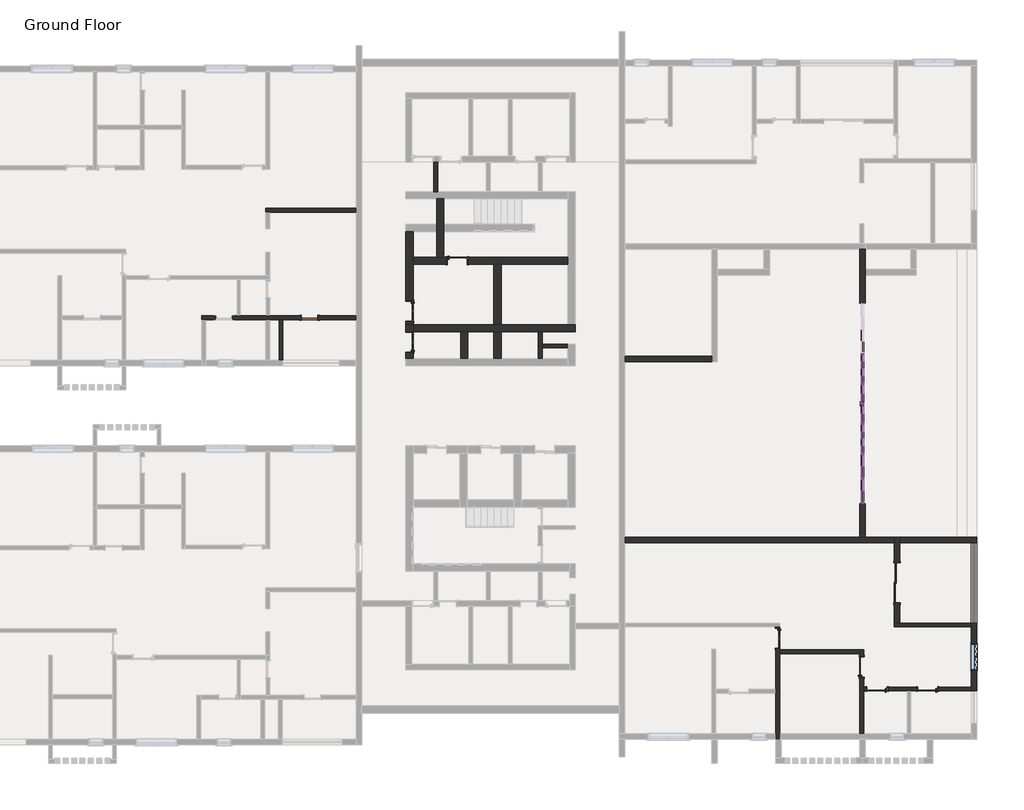
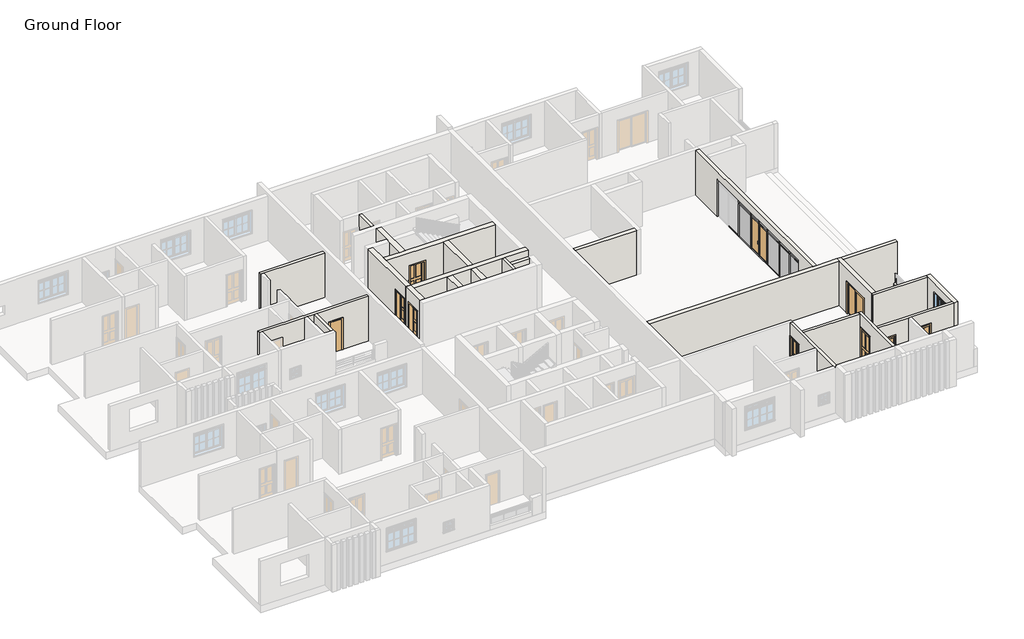
# One storey, part 4 of 9: 32 members, 26 walls, 10 doors, 10 plates, 1 window.
"""IFC4 building model written with IfcOpenShell, lengths in millimetres."""

from ifc_helpers import new_model, si_unit, origin, origin_with_axes, place, context, project, spatial, polyline, outline, extrude, faceted_brep, transform, mapped, element, save
from components import door_curtain_wall_double_storefront_door_curtain_wall_double_c727979e, door_double_sliding_6_7f701685, door_interior_single_4_panel_wood_3_x_7_bed_room_doors_9f8eaeea, door_interior_single_4_panel_wood_3_x_7_bed_room_doors_791c550c, door_interior_single_4_panel_wood_3_x_7_bed_room_doors_8c54f457, door_0af0cdd0, member_75d1e245, member_7db1855a, member_d2e7e466, member_80bb9b3a, member_1988fdfd, member_d37749d9, member_bf0a6844, member_74e81316, member_697f972d, member_78934672, member_3c3dc66a, member_222163d1, member_5cd4c5ac, member_860c46db, system_panel_glazed_fbb6c980, system_panel_glazed_ad1fd27a, system_panel_glazed_1d13bf28, system_panel_glazed_6ba3ac31, system_panel_glazed_eda788cd, system_panel_glazed_2483beae, system_panel_glazed_98578528, window_casement_double_awning_double_4_x_5_window_c6f36ef5

model = new_model("IFC4")

# Units and contexts
model_context = context("Model", 3, world=origin())
ifc_project = project(units=[si_unit("LENGTHUNIT", "METRE", prefix="MILLI")], contexts=[model_context])

# Site, building, storey
site = spatial("IfcSite", under=ifc_project)
building = spatial("IfcBuilding", under=site)
storey = spatial("IfcBuildingStorey", under=building, Name="Ground Floor", Elevation=0.0)

# Doors
placement = place(None, origin())
door_curtain_wall_double_storefront_door_curtain_wall_double_shape = door_curtain_wall_double_storefront_door_curtain_wall_double_c727979e(model_context)
element("IfcDoor", 1, ObjectType="Door-Curtain-Wall-Double-Storefront : Door-Curtain-Wall-Double-Storefront", at=placement, inside=storey, context=model_context, shape_type="MappedRepresentation", body=[
    mapped(door_curtain_wall_double_storefront_door_curtain_wall_double_shape, transform((26870.0546318, 13572.234892, 63.5), x_axis=(0.0, 1.0, 0.0), y_axis=(-1.0, 0.0, 0.0), z_axis=(0.0, 0.0, 1.0))),
])
door_double_sliding_6_shape = door_double_sliding_6_7f701685(model_context)
element("IfcDoor", 2, ObjectType="Door-Double-Sliding : 6'", at=placement, inside=storey, context=model_context, shape_type="MappedRepresentation", body=[
    mapped(door_double_sliding_6_shape, transform((28571.8546318, 5393.434892, 0.0), x_axis=(0.0, 1.0, 0.0), y_axis=(-1.0, 0.0, 0.0), z_axis=(0.0, 0.0, 1.0))),
])
door_interior_single_4_panel_wood_3_x_7_bed_room_doors_shape = door_interior_single_4_panel_wood_3_x_7_bed_room_doors_9f8eaeea(model_context)
element("IfcDoor", 3, ObjectType="Door-Interior-Single-4_Panel-Wood : 3' x 7' Bed Room Doors", at=placement, inside=storey, context=model_context, shape_type="MappedRepresentation", body=[
    mapped(door_interior_single_4_panel_wood_3_x_7_bed_room_doors_shape, transform((22999.7296318, 2866.134892, 0.0), x_axis=(0.0, -1.0, 0.0), y_axis=(1.0, 0.0, 0.0), z_axis=(0.0, 0.0, 1.0))),
])
element("IfcDoor", 4, ObjectType="Door-Interior-Single-4_Panel-Wood : 3' x 7' Bed Room Doors", at=placement, inside=storey, context=model_context, shape_type="MappedRepresentation", body=[
    mapped(door_interior_single_4_panel_wood_3_x_7_bed_room_doors_shape, transform((26828.7796318, 1558.034892, 0.0), x_axis=(0.0, 1.0, 0.0), y_axis=(-1.0, 0.0, 0.0), z_axis=(0.0, 0.0, 1.0))),
])
element("IfcDoor", 5, ObjectType="Door-Interior-Single-4_Panel-Wood : 3' x 7' Bed Room Doors", at=placement, inside=storey, context=model_context, shape_type="MappedRepresentation", body=[
    mapped(door_interior_single_4_panel_wood_3_x_7_bed_room_doors_shape, transform((27530.4546318, 551.559892, 0.0), x_axis=(-1.0, 0.0, 0.0), y_axis=(0.0, -1.0, 0.0), z_axis=(0.0, 0.0, 1.0))),
])
element("IfcDoor", 6, ObjectType="Door-Interior-Single-4_Panel-Wood : 3' x 7' Bed Room Doors", at=placement, inside=storey, context=model_context, shape_type="MappedRepresentation", body=[
    mapped(door_interior_single_4_panel_wood_3_x_7_bed_room_doors_shape, transform((29841.8546318, 551.559892, 0.0), x_axis=(-1.0, 0.0, 0.0), y_axis=(0.0, -1.0, 0.0), z_axis=(0.0, 0.0, 1.0))),
])
door_interior_single_4_panel_wood_3_x_7_bed_room_doors_2_shape = door_interior_single_4_panel_wood_3_x_7_bed_room_doors_791c550c(model_context)
element("IfcDoor", 7, ObjectType="Door-Interior-Single-4_Panel-Wood : 3' x 7' Bed Room Doors", at=placement, inside=storey, context=model_context, shape_type="MappedRepresentation", body=[
    mapped(door_interior_single_4_panel_wood_3_x_7_bed_room_doors_2_shape, transform((6210.3296318, 17788.634892, 0.0), x_axis=(0.0, -1.0, 0.0), y_axis=(1.0, 0.0, 0.0), z_axis=(0.0, 0.0, 1.0))),
])
element("IfcDoor", 8, ObjectType="Door-Interior-Single-4_Panel-Wood : 3' x 7' Bed Room Doors", at=placement, inside=storey, context=model_context, shape_type="MappedRepresentation", body=[
    mapped(door_interior_single_4_panel_wood_3_x_7_bed_room_doors_2_shape, transform((8378.8546318, 20090.509892, 0.0), x_axis=(1.0, 0.0, 0.0), y_axis=(0.0, 1.0, 0.0), z_axis=(0.0, 0.0, 1.0))),
])
door_interior_single_4_panel_wood_3_x_7_bed_room_doors_3_shape = door_interior_single_4_panel_wood_3_x_7_bed_room_doors_8c54f457(model_context)
element("IfcDoor", 9, ObjectType="Door-Interior-Single-4_Panel-Wood : 3' x 7' Bed Room Doors", at=placement, inside=storey, context=model_context, shape_type="MappedRepresentation", body=[
    mapped(door_interior_single_4_panel_wood_3_x_7_bed_room_doors_3_shape, transform((6210.3296318, 16366.234892, 0.0), x_axis=(0.0, 1.0, 0.0), y_axis=(-1.0, 0.0, 0.0), z_axis=(0.0, 0.0, 1.0))),
])
door_shape = door_0af0cdd0(model_context)
element("IfcDoor", 10, ObjectType="Single-Flush : 30\" x 80\"", at=placement, inside=storey, context=model_context, shape_type="MappedRepresentation", body=[
    mapped(door_shape, transform((1647.8546318, 17496.534892, 0.0), x_axis=(-1.0, 0.0, 0.0), y_axis=(0.0, -1.0, 0.0), z_axis=(0.0, 0.0, 1.0))),
])

# Members
member_shape = member_75d1e245(model_context)
element("IfcMember", 11, ObjectType="Rectangular Mullion : 2.5\" x 5\" rectangular", at=placement, inside=storey, context=model_context, shape_type="MappedRepresentation", body=[
    mapped(member_shape, transform((26870.0546318, 14486.634892, 2286.0), x_axis=(0.0, 1.0, 0.0), y_axis=(1.0, 0.0, 0.0), z_axis=(0.0, 0.0, -1.0))),
])
element("IfcMember", 12, ObjectType="Rectangular Mullion : 2.5\" x 5\" rectangular", at=placement, inside=storey, context=model_context, shape_type="MappedRepresentation", body=[
    mapped(member_shape, transform((26870.0546318, 12657.834892, 2286.0), x_axis=(0.0, 1.0, 0.0), y_axis=(1.0, 0.0, 0.0), z_axis=(0.0, 0.0, -1.0))),
])
element("IfcMember", 13, ObjectType="Rectangular Mullion : 2.5\" x 5\" rectangular", at=placement, inside=storey, context=model_context, shape_type="MappedRepresentation", body=[
    mapped(member_shape, transform((26870.0546318, 11286.234892, 2286.0), x_axis=(0.0, 1.0, 0.0), y_axis=(1.0, 0.0, 0.0), z_axis=(0.0, 0.0, -1.0))),
])
element("IfcMember", 14, ObjectType="Rectangular Mullion : 2.5\" x 5\" rectangular", at=placement, inside=storey, context=model_context, shape_type="MappedRepresentation", body=[
    mapped(member_shape, transform((26870.0546318, 10143.234892, 2286.0), x_axis=(0.0, 1.0, 0.0), y_axis=(1.0, 0.0, 0.0), z_axis=(0.0, 0.0, -1.0))),
])
element("IfcMember", 15, ObjectType="Rectangular Mullion : 2.5\" x 5\" rectangular", at=placement, inside=storey, context=model_context, shape_type="MappedRepresentation", body=[
    mapped(member_shape, transform((26870.0546318, 15858.234892, 2286.0), x_axis=(0.0, 1.0, 0.0), y_axis=(1.0, 0.0, 0.0), z_axis=(0.0, 0.0, -1.0))),
])
member_2_shape = member_7db1855a(model_context)
element("IfcMember", 16, ObjectType="Rectangular Mullion : 2.5\" x 5\" rectangular", at=placement, inside=storey, context=model_context, shape_type="MappedRepresentation", body=[
    mapped(member_2_shape, transform((26870.0546318, 13540.484892, 2286.0), x_axis=(0.0, 0.0, 1.0), y_axis=(1.0, 0.0, 0.0), z_axis=(0.0, 1.0, 0.0))),
])
element("IfcMember", 17, ObjectType="Rectangular Mullion : 2.5\" x 5\" rectangular", at=placement, inside=storey, context=model_context, shape_type="MappedRepresentation", body=[
    mapped(member_2_shape, transform((26870.0546318, 14454.884892, 2286.0), x_axis=(0.0, 0.0, 1.0), y_axis=(1.0, 0.0, 0.0), z_axis=(0.0, 1.0, 0.0))),
])
member_3_shape = member_d2e7e466(model_context)
element("IfcMember", 18, ObjectType="Rectangular Mullion : 2.5\" x 5\" rectangular", at=placement, inside=storey, context=model_context, shape_type="MappedRepresentation", body=[
    mapped(member_3_shape, transform((26870.0546318, 14454.884892, 2590.8), x_axis=(0.0, 0.0, 1.0), y_axis=(1.0, 0.0, 0.0), z_axis=(0.0, 1.0, 0.0))),
])
element("IfcMember", 19, ObjectType="Rectangular Mullion : 2.5\" x 5\" rectangular", at=placement, inside=storey, context=model_context, shape_type="MappedRepresentation", body=[
    mapped(member_3_shape, transform((26870.0546318, 13540.484892, 2590.8), x_axis=(0.0, 0.0, 1.0), y_axis=(1.0, 0.0, 0.0), z_axis=(0.0, 1.0, 0.0))),
])
member_4_shape = member_80bb9b3a(model_context)
element("IfcMember", 20, ObjectType="Rectangular Mullion : 2.5\" x 5\" rectangular", at=placement, inside=storey, context=model_context, shape_type="MappedRepresentation", body=[
    mapped(member_4_shape, transform((26870.0546318, 13572.234892, 2254.25), x_axis=(0.0, 1.0, 0.0), y_axis=(1.0, 0.0, 0.0), z_axis=(0.0, 0.0, -1.0))),
])
member_5_shape = member_1988fdfd(model_context)
element("IfcMember", 21, ObjectType="Rectangular Mullion : 2.5\" x 5\" rectangular", at=placement, inside=storey, context=model_context, shape_type="MappedRepresentation", body=[
    mapped(member_5_shape, transform((26870.0546318, 15826.484892, 2286.0), x_axis=(0.0, 0.0, 1.0), y_axis=(1.0, 0.0, 0.0), z_axis=(0.0, 1.0, 0.0))),
])
element("IfcMember", 22, ObjectType="Rectangular Mullion : 2.5\" x 5\" rectangular", at=placement, inside=storey, context=model_context, shape_type="MappedRepresentation", body=[
    mapped(member_5_shape, transform((26870.0546318, 12626.084892, 2286.0), x_axis=(0.0, 0.0, 1.0), y_axis=(1.0, 0.0, 0.0), z_axis=(0.0, 1.0, 0.0))),
])
member_6_shape = member_d37749d9(model_context)
element("IfcMember", 23, ObjectType="Rectangular Mullion : 2.5\" x 5\" rectangular", at=placement, inside=storey, context=model_context, shape_type="MappedRepresentation", body=[
    mapped(member_6_shape, transform((26870.0546318, 12626.084892, 2590.8), x_axis=(0.0, 0.0, 1.0), y_axis=(1.0, 0.0, 0.0), z_axis=(0.0, 1.0, 0.0))),
])
element("IfcMember", 24, ObjectType="Rectangular Mullion : 2.5\" x 5\" rectangular", at=placement, inside=storey, context=model_context, shape_type="MappedRepresentation", body=[
    mapped(member_6_shape, transform((26870.0546318, 15826.484892, 2590.8), x_axis=(0.0, 0.0, 1.0), y_axis=(1.0, 0.0, 0.0), z_axis=(0.0, 1.0, 0.0))),
])
member_7_shape = member_bf0a6844(model_context)
element("IfcMember", 25, ObjectType="Rectangular Mullion : 2.5\" x 5\" rectangular", at=placement, inside=storey, context=model_context, shape_type="MappedRepresentation", body=[
    mapped(member_7_shape, transform((26870.0546318, 11254.484892, 2286.0), x_axis=(0.0, 0.0, 1.0), y_axis=(1.0, 0.0, 0.0), z_axis=(0.0, 1.0, 0.0))),
])
member_8_shape = member_74e81316(model_context)
element("IfcMember", 26, ObjectType="Rectangular Mullion : 2.5\" x 5\" rectangular", at=placement, inside=storey, context=model_context, shape_type="MappedRepresentation", body=[
    mapped(member_8_shape, transform((26870.0546318, 11254.484892, 2590.8), x_axis=(0.0, 0.0, 1.0), y_axis=(1.0, 0.0, 0.0), z_axis=(0.0, 1.0, 0.0))),
])
member_9_shape = member_697f972d(model_context)
element("IfcMember", 27, ObjectType="Rectangular Mullion : 2.5\" x 5\" rectangular", at=placement, inside=storey, context=model_context, shape_type="MappedRepresentation", body=[
    mapped(member_9_shape, transform((26870.0546318, 10111.484892, 2286.0), x_axis=(0.0, 0.0, 1.0), y_axis=(1.0, 0.0, 0.0), z_axis=(0.0, 1.0, 0.0))),
])
member_10_shape = member_78934672(model_context)
element("IfcMember", 28, ObjectType="Rectangular Mullion : 2.5\" x 5\" rectangular", at=placement, inside=storey, context=model_context, shape_type="MappedRepresentation", body=[
    mapped(member_10_shape, transform((26870.0546318, 10111.484892, 2590.8), x_axis=(0.0, 0.0, 1.0), y_axis=(1.0, 0.0, 0.0), z_axis=(0.0, 1.0, 0.0))),
])
member_11_shape = member_3c3dc66a(model_context)
element("IfcMember", 29, ObjectType="Rectangular Mullion : 2.5\" x 5\" rectangular", at=placement, inside=storey, context=model_context, shape_type="MappedRepresentation", body=[
    mapped(member_11_shape, transform((26870.0546318, 9000.234892, 2590.8), x_axis=(0.0, -1.0, 0.0), y_axis=(1.0, 0.0, 0.0), z_axis=(0.0, 0.0, 1.0))),
])
member_12_shape = member_222163d1(model_context)
element("IfcMember", 30, ObjectType="Rectangular Mullion : 2.5\" x 5\" rectangular", at=placement, inside=storey, context=model_context, shape_type="MappedRepresentation", body=[
    mapped(member_12_shape, transform((26870.0546318, 14486.634892, 0.0), x_axis=(0.0, 1.0, 0.0), y_axis=(1.0, 0.0, 0.0), z_axis=(0.0, 0.0, -1.0))),
])
element("IfcMember", 31, ObjectType="Rectangular Mullion : 2.5\" x 5\" rectangular", at=placement, inside=storey, context=model_context, shape_type="MappedRepresentation", body=[
    mapped(member_12_shape, transform((26870.0546318, 12657.834892, 0.0), x_axis=(0.0, 1.0, 0.0), y_axis=(1.0, 0.0, 0.0), z_axis=(0.0, 0.0, -1.0))),
])
element("IfcMember", 32, ObjectType="Rectangular Mullion : 2.5\" x 5\" rectangular", at=placement, inside=storey, context=model_context, shape_type="MappedRepresentation", body=[
    mapped(member_12_shape, transform((26870.0546318, 11286.234892, 0.0), x_axis=(0.0, 1.0, 0.0), y_axis=(1.0, 0.0, 0.0), z_axis=(0.0, 0.0, -1.0))),
])
element("IfcMember", 33, ObjectType="Rectangular Mullion : 2.5\" x 5\" rectangular", at=placement, inside=storey, context=model_context, shape_type="MappedRepresentation", body=[
    mapped(member_12_shape, transform((26870.0546318, 10143.234892, 0.0), x_axis=(0.0, 1.0, 0.0), y_axis=(1.0, 0.0, 0.0), z_axis=(0.0, 0.0, -1.0))),
])
element("IfcMember", 34, ObjectType="Rectangular Mullion : 2.5\" x 5\" rectangular", at=placement, inside=storey, context=model_context, shape_type="MappedRepresentation", body=[
    mapped(member_12_shape, transform((26870.0546318, 15858.234892, 0.0), x_axis=(0.0, 1.0, 0.0), y_axis=(1.0, 0.0, 0.0), z_axis=(0.0, 0.0, -1.0))),
])
element("IfcMember", 35, ObjectType="Rectangular Mullion : 2.5\" x 5\" rectangular", at=placement, inside=storey, context=model_context, shape_type="MappedRepresentation", body=[
    mapped(member_8_shape, transform((26870.0546318, 10174.984892, 0.0), x_axis=(0.0, 0.0, -1.0), y_axis=(1.0, 0.0, 0.0), z_axis=(0.0, -1.0, 0.0))),
])
element("IfcMember", 36, ObjectType="Rectangular Mullion : 2.5\" x 5\" rectangular", at=placement, inside=storey, context=model_context, shape_type="MappedRepresentation", body=[
    mapped(member_8_shape, transform((26870.0546318, 15889.984892, 0.0), x_axis=(0.0, 0.0, -1.0), y_axis=(1.0, 0.0, 0.0), z_axis=(0.0, -1.0, 0.0))),
])
element("IfcMember", 37, ObjectType="Rectangular Mullion : 2.5\" x 5\" rectangular", at=placement, inside=storey, context=model_context, shape_type="MappedRepresentation", body=[
    mapped(member_6_shape, transform((26870.0546318, 14518.384892, 0.0), x_axis=(0.0, 0.0, -1.0), y_axis=(1.0, 0.0, 0.0), z_axis=(0.0, -1.0, 0.0))),
])
element("IfcMember", 38, ObjectType="Rectangular Mullion : 2.5\" x 5\" rectangular", at=placement, inside=storey, context=model_context, shape_type="MappedRepresentation", body=[
    mapped(member_6_shape, transform((26870.0546318, 11317.984892, 0.0), x_axis=(0.0, 0.0, -1.0), y_axis=(1.0, 0.0, 0.0), z_axis=(0.0, -1.0, 0.0))),
])
member_13_shape = member_5cd4c5ac(model_context)
element("IfcMember", 39, ObjectType="Rectangular Mullion : 2.5\" x 5\" rectangular", at=placement, inside=storey, context=model_context, shape_type="MappedRepresentation", body=[
    mapped(member_13_shape, transform((26870.0546318, 12689.584892, 0.0), x_axis=(0.0, 0.0, -1.0), y_axis=(1.0, 0.0, 0.0), z_axis=(0.0, -1.0, 0.0))),
])
element("IfcMember", 40, ObjectType="Rectangular Mullion : 2.5\" x 5\" rectangular", at=placement, inside=storey, context=model_context, shape_type="MappedRepresentation", body=[
    mapped(member_10_shape, transform((26870.0546318, 9063.734892, 0.0), x_axis=(0.0, 0.0, -1.0), y_axis=(1.0, 0.0, 0.0), z_axis=(0.0, -1.0, 0.0))),
])
element("IfcMember", 41, ObjectType="Rectangular Mullion : 2.5\" x 5\" rectangular", at=placement, inside=storey, context=model_context, shape_type="MappedRepresentation", body=[
    mapped(member_13_shape, transform((26870.0546318, 13572.234892, 0.0), x_axis=(0.0, 0.0, -1.0), y_axis=(1.0, 0.0, 0.0), z_axis=(0.0, -1.0, 0.0))),
])
member_14_shape = member_860c46db(model_context)
element("IfcMember", 42, ObjectType="Rectangular Mullion : 2.5\" x 5\" rectangular", at=placement, inside=storey, context=model_context, shape_type="MappedRepresentation", body=[
    mapped(member_14_shape, transform((26870.0546318, 9000.234892, 2286.0), x_axis=(0.0, -1.0, 0.0), y_axis=(1.0, 0.0, 0.0), z_axis=(0.0, 0.0, 1.0))),
])

# Plates
system_panel_glazed_shape = system_panel_glazed_fbb6c980(model_context)
element("IfcPlate", 43, ObjectType="System Panel : Glazed", at=placement, inside=storey, context=model_context, shape_type="MappedRepresentation", body=[
    mapped(system_panel_glazed_shape, transform((26870.0546318, 13115.034892, 2317.75), x_axis=(0.0, 1.0, 0.0), y_axis=(-1.0, 0.0, 0.0), z_axis=(0.0, 0.0, 1.0))),
])
element("IfcPlate", 44, ObjectType="System Panel : Glazed", at=placement, inside=storey, context=model_context, shape_type="MappedRepresentation", body=[
    mapped(system_panel_glazed_shape, transform((26870.0546318, 14029.434892, 2317.75), x_axis=(0.0, 1.0, 0.0), y_axis=(-1.0, 0.0, 0.0), z_axis=(0.0, 0.0, 1.0))),
])
system_panel_glazed_2_shape = system_panel_glazed_ad1fd27a(model_context)
element("IfcPlate", 45, ObjectType="System Panel : Glazed", at=placement, inside=storey, context=model_context, shape_type="MappedRepresentation", body=[
    mapped(system_panel_glazed_2_shape, transform((26870.0546318, 11972.034892, 2317.75), x_axis=(0.0, 1.0, 0.0), y_axis=(-1.0, 0.0, 0.0), z_axis=(0.0, 0.0, 1.0))),
])
element("IfcPlate", 46, ObjectType="System Panel : Glazed", at=placement, inside=storey, context=model_context, shape_type="MappedRepresentation", body=[
    mapped(system_panel_glazed_2_shape, transform((26870.0546318, 15172.434892, 2317.75), x_axis=(0.0, 1.0, 0.0), y_axis=(-1.0, 0.0, 0.0), z_axis=(0.0, 0.0, 1.0))),
])
system_panel_glazed_3_shape = system_panel_glazed_1d13bf28(model_context)
element("IfcPlate", 47, ObjectType="System Panel : Glazed", at=placement, inside=storey, context=model_context, shape_type="MappedRepresentation", body=[
    mapped(system_panel_glazed_3_shape, transform((26870.0546318, 10714.734892, 2317.75), x_axis=(0.0, 1.0, 0.0), y_axis=(-1.0, 0.0, 0.0), z_axis=(0.0, 0.0, 1.0))),
])
system_panel_glazed_4_shape = system_panel_glazed_6ba3ac31(model_context)
element("IfcPlate", 48, ObjectType="System Panel : Glazed", at=placement, inside=storey, context=model_context, shape_type="MappedRepresentation", body=[
    mapped(system_panel_glazed_4_shape, transform((26870.0546318, 9587.609892, 2317.75), x_axis=(0.0, 1.0, 0.0), y_axis=(-1.0, 0.0, 0.0), z_axis=(0.0, 0.0, 1.0))),
])
system_panel_glazed_5_shape = system_panel_glazed_eda788cd(model_context)
element("IfcPlate", 49, ObjectType="System Panel : Glazed", at=placement, inside=storey, context=model_context, shape_type="MappedRepresentation", body=[
    mapped(system_panel_glazed_5_shape, transform((26870.0546318, 9587.609892, 63.5), x_axis=(0.0, 1.0, 0.0), y_axis=(-1.0, 0.0, 0.0), z_axis=(0.0, 0.0, 1.0))),
])
system_panel_glazed_6_shape = system_panel_glazed_2483beae(model_context)
element("IfcPlate", 50, ObjectType="System Panel : Glazed", at=placement, inside=storey, context=model_context, shape_type="MappedRepresentation", body=[
    mapped(system_panel_glazed_6_shape, transform((26870.0546318, 11972.034892, 63.5), x_axis=(0.0, 1.0, 0.0), y_axis=(-1.0, 0.0, 0.0), z_axis=(0.0, 0.0, 1.0))),
])
element("IfcPlate", 51, ObjectType="System Panel : Glazed", at=placement, inside=storey, context=model_context, shape_type="MappedRepresentation", body=[
    mapped(system_panel_glazed_6_shape, transform((26870.0546318, 15172.434892, 63.5), x_axis=(0.0, 1.0, 0.0), y_axis=(-1.0, 0.0, 0.0), z_axis=(0.0, 0.0, 1.0))),
])
system_panel_glazed_7_shape = system_panel_glazed_98578528(model_context)
element("IfcPlate", 52, ObjectType="System Panel : Glazed", at=placement, inside=storey, context=model_context, shape_type="MappedRepresentation", body=[
    mapped(system_panel_glazed_7_shape, transform((26870.0546318, 10714.734892, 63.5), x_axis=(0.0, 1.0, 0.0), y_axis=(-1.0, 0.0, 0.0), z_axis=(0.0, 0.0, 1.0))),
])

# Walls
element("IfcWall", 53, ObjectType="12\" EXTERIOR WALL", at=placement, inside=storey, context=model_context, shape_type="Brep", body=[
    faceted_brep([(6372.2546318, 16848.834892, 0.0), (6372.2546318, 17179.034892, 0.0), (6372.2546318, 17179.034892, 3048.0), (6372.2546318, 16848.834892, 3048.0), (6372.2546318, 15629.634892, 3048.0), (6372.2546318, 15629.634892, 0.0), (6372.2546318, 15883.634892, 0.0), (6372.2546318, 15883.634892, 2159.0), (6372.2546318, 16848.834892, 2159.0), (6042.0546318, 17179.034892, 0.0), (6042.0546318, 16848.834892, 0.0), (6042.0546318, 16848.834892, 2159.0), (6042.0546318, 15883.634892, 2159.0), (6042.0546318, 15883.634892, 0.0), (6042.0546318, 15629.634892, 0.0), (6042.0546318, 15629.634892, 3048.0), (6042.0546318, 17179.034892, 3048.0)], [[[0, 1, 2, 3, 4, 5, 6, 7, 8]], [[9, 10, 11, 12, 13, 14, 15, 16]], [[5, 14, 13, 6]], [[9, 1, 0, 10]], [[14, 5, 4, 15]], [[1, 9, 16, 2]], [[4, 3, 2, 16, 15]], [[8, 11, 10, 0]], [[11, 8, 7, 12]], [[12, 7, 6, 13]]]),
])
element("IfcWall", 54, ObjectType="12\" EXTERIOR WALL", at=placement, inside=storey, context=model_context, shape_type="Brep", body=[
    faceted_brep([(6372.2546318, 16848.834892, 0.0), (8531.2546318, 16848.834892, 0.0), (8861.4546318, 16848.834892, 0.0), (10055.2546318, 16848.834892, 0.0), (10385.4546318, 16848.834892, 0.0), (12087.2546318, 16848.834892, 0.0), (12265.0546318, 16848.834892, 0.0), (13763.6546318, 16848.834892, 0.0), (13763.6546318, 16848.834892, 3048.0), (12265.0546318, 16848.834892, 3048.0), (12087.2546318, 16848.834892, 3048.0), (6372.2546318, 16848.834892, 3048.0), (13763.6546318, 17179.034892, 0.0), (13433.4546318, 17179.034892, 0.0), (10385.4546318, 17179.034892, 0.0), (10055.2546318, 17179.034892, 0.0), (6372.2546318, 17179.034892, 0.0), (6372.2546318, 17179.034892, 3048.0), (13763.6546318, 17179.034892, 3048.0)], [[[0, 1, 2, 3, 4, 5, 6, 7, 8, 9, 10, 11]], [[12, 13, 14, 15, 16, 17, 18]], [[7, 6, 5, 4, 3, 2, 1, 0, 16, 15, 14, 13, 12]], [[16, 0, 11, 17]], [[7, 12, 18, 8]], [[11, 10, 9, 8, 18, 17]]]),
])
element("IfcWall", 55, ObjectType="12\" EXTERIOR WALL", at=placement, inside=storey, context=model_context, shape_type="SweptSolid", body=[
    extrude(outline(polyline([(10055.2546318, 15629.634892), (10055.2546318, 16848.834892), (10385.4546318, 16848.834892), (10385.4546318, 15629.634892), (10055.2546318, 15629.634892)])), origin_with_axes(), (0.0, 0.0, 1.0), 3048.0),
])
element("IfcWall", 56, ObjectType="12\" EXTERIOR WALL", at=placement, inside=storey, context=model_context, shape_type="SweptSolid", body=[
    extrude(outline(polyline([(8531.2546318, 15629.634892), (8531.2546318, 16848.834892), (8861.4546318, 16848.834892), (8861.4546318, 15629.634892), (8531.2546318, 15629.634892)])), origin_with_axes(), (0.0, 0.0, 1.0), 3048.0),
])
element("IfcWall", 57, ObjectType="12\" EXTERIOR WALL", at=placement, inside=storey, context=model_context, shape_type="Brep", body=[
    faceted_brep([(13433.4546318, 20252.434892, 0.0), (8861.4546318, 20252.434892, 0.0), (8861.4546318, 20252.434892, 2159.0), (7896.2546318, 20252.434892, 2159.0), (7896.2546318, 20252.434892, 0.0), (7769.2546318, 20252.434892, 0.0), (7439.0546318, 20252.434892, 0.0), (6372.2546318, 20252.434892, 0.0), (6372.2546318, 20252.434892, 3048.0), (7439.0546318, 20252.434892, 3048.0), (7769.2546318, 20252.434892, 3048.0), (9166.2546318, 20252.434892, 3048.0), (13433.4546318, 20252.434892, 3048.0), (8861.4546318, 19922.234892, 0.0), (10055.2546318, 19922.234892, 0.0), (10385.4546318, 19922.234892, 0.0), (13433.4546318, 19922.234892, 0.0), (13433.4546318, 19922.234892, 3048.0), (10385.4546318, 19922.234892, 3048.0), (10055.2546318, 19922.234892, 3048.0), (6372.2546318, 19922.234892, 3048.0), (6372.2546318, 19922.234892, 0.0), (7896.2546318, 19922.234892, 0.0), (7896.2546318, 19922.234892, 2159.0), (8861.4546318, 19922.234892, 2159.0)], [[[0, 1, 2, 3, 4, 5, 6, 7, 8, 9, 10, 11, 12]], [[13, 14, 15, 16, 17, 18, 19, 20, 21, 22, 23, 24]], [[0, 16, 15, 14, 13, 1]], [[21, 7, 6, 5, 4, 22]], [[16, 0, 12, 17]], [[7, 21, 20, 8]], [[12, 11, 10, 9, 8, 20, 19, 18, 17]], [[24, 2, 1, 13]], [[2, 24, 23, 3]], [[3, 23, 22, 4]]]),
])
element("IfcWall", 58, ObjectType="12\" EXTERIOR WALL", at=placement, inside=storey, context=model_context, shape_type="SweptSolid", body=[
    extrude(outline(polyline([(10055.2546318, 17179.034892), (10055.2546318, 19922.234892), (10385.4546318, 19922.234892), (10385.4546318, 17179.034892), (10055.2546318, 17179.034892)])), origin_with_axes(), (0.0, 0.0, 1.0), 3048.0),
])
element("IfcWall", 59, ObjectType="12\" EXTERIOR WALL", at=placement, inside=storey, context=model_context, shape_type="Brep", body=[
    faceted_brep([(6042.0546318, 17306.034892, 0.0), (6042.0546318, 17179.034892, 0.0), (6042.0546318, 17179.034892, 3048.0), (6042.0546318, 21420.834892, 3048.0), (6042.0546318, 21420.834892, 0.0), (6042.0546318, 18271.234892, 0.0), (6042.0546318, 18271.234892, 2159.0), (6042.0546318, 17306.034892, 2159.0), (6372.2546318, 17179.034892, 0.0), (6372.2546318, 17306.034892, 0.0), (6372.2546318, 17306.034892, 2159.0), (6372.2546318, 18271.234892, 2159.0), (6372.2546318, 18271.234892, 0.0), (6372.2546318, 19922.234892, 0.0), (6372.2546318, 20252.434892, 0.0), (6372.2546318, 21420.834892, 0.0), (6372.2546318, 21420.834892, 3048.0), (6372.2546318, 20252.434892, 3048.0), (6372.2546318, 19922.234892, 3048.0), (6372.2546318, 17179.034892, 3048.0)], [[[0, 1, 2, 3, 4, 5, 6, 7]], [[8, 9, 10, 11, 12, 13, 14, 15, 16, 17, 18, 19]], [[8, 1, 0, 9]], [[4, 15, 14, 13, 12, 5]], [[1, 8, 19, 2]], [[15, 4, 3, 16]], [[3, 2, 19, 18, 17, 16]], [[7, 10, 9, 0]], [[10, 7, 6, 11]], [[11, 6, 5, 12]]]),
])
element("IfcWall", 60, ObjectType="12\" EXTERIOR WALL", at=placement, inside=storey, context=model_context, shape_type="Brep", body=[
    faceted_brep([(7439.0546318, 22919.434892, 0.0), (7439.0546318, 21751.034892, 0.0), (7439.0546318, 21420.834892, 0.0), (7439.0546318, 20252.434892, 0.0), (7439.0546318, 20252.434892, 3048.0), (7439.0546318, 21420.834892, 3048.0), (7439.0546318, 21751.034892, 3048.0), (7439.0546318, 22919.434892, 3048.0), (7769.2546318, 20252.434892, 0.0), (7769.2546318, 21420.834892, 0.0), (7769.2546318, 21751.034892, 0.0), (7769.2546318, 22919.434892, 0.0), (7769.2546318, 22919.434892, 3048.0), (7769.2546318, 21751.034892, 3048.0), (7769.2546318, 21420.834892, 3048.0), (7769.2546318, 20252.434892, 3048.0)], [[[0, 1, 2, 3, 4, 5, 6, 7]], [[8, 9, 10, 11, 12, 13, 14, 15]], [[3, 2, 1, 0, 11, 10, 9, 8]], [[3, 8, 15, 4]], [[7, 6, 5, 4, 15, 14, 13, 12]], [[11, 0, 7, 12]]]),
])
element("IfcWall", 61, ObjectType="6\" INTERIOR WALL", at=placement, inside=storey, context=model_context, shape_type="Brep", body=[
    faceted_brep([(12087.2546318, 16848.834892, 0.0), (12087.2546318, 15629.634892, 0.0), (12087.2546318, 15629.634892, 3048.0), (12087.2546318, 16848.834892, 3048.0), (12265.0546318, 15629.634892, 0.0), (12265.0546318, 16112.234892, 0.0), (12265.0546318, 16290.034892, 0.0), (12265.0546318, 16848.834892, 0.0), (12265.0546318, 16848.834892, 3048.0), (12265.0546318, 16290.034892, 3048.0), (12265.0546318, 16112.234892, 3048.0), (12265.0546318, 15629.634892, 3048.0)], [[[0, 1, 2, 3]], [[4, 5, 6, 7, 8, 9, 10, 11]], [[1, 0, 7, 6, 5, 4]], [[1, 4, 11, 2]], [[7, 0, 3, 8]], [[3, 2, 11, 10, 9, 8]]]),
])
element("IfcWall", 62, ObjectType="6\" INTERIOR WALL", at=placement, inside=storey, context=model_context, shape_type="SweptSolid", body=[
    extrude(outline(polyline([(12265.0546318, 16290.034892), (13433.4546318, 16290.034892), (13433.4546318, 16112.234892), (12265.0546318, 16112.234892), (12265.0546318, 16290.034892)])), origin_with_axes(), (0.0, 0.0, 1.0), 3048.0),
])
element("IfcWall", 63, ObjectType="6\" INTERIOR WALL", at=placement, inside=storey, context=model_context, shape_type="Brep", body=[
    faceted_brep([(-1882.7453682, 17585.434892, 0.0), (-1882.7453682, 17585.434892, 2133.6), (-2644.7453682, 17585.434892, 2133.6), (-2644.7453682, 17585.434892, 0.0), (-3279.7453682, 17585.434892, 0.0), (-3279.7453682, 17585.434892, 3048.0), (-1654.1453682, 17585.434892, 3048.0), (-1514.4453682, 17585.434892, 3048.0), (-320.6453682, 17585.434892, 3048.0), (-180.9453682, 17585.434892, 3048.0), (3781.4546318, 17585.434892, 3048.0), (3781.4546318, 17585.434892, 0.0), (2028.8546318, 17585.434892, 0.0), (2028.8546318, 17585.434892, 2133.6), (1266.8546318, 17585.434892, 2133.6), (1266.8546318, 17585.434892, 0.0), (-180.9453682, 17585.434892, 0.0), (-320.6453682, 17585.434892, 0.0), (-1514.4453682, 17585.434892, 0.0), (-1654.1453682, 17585.434892, 0.0), (-1882.7453682, 17407.634892, 2133.6), (-1882.7453682, 17407.634892, 0.0), (-358.7453682, 17407.634892, 0.0), (-180.9453682, 17407.634892, 0.0), (250.8546318, 17407.634892, 0.0), (428.6546318, 17407.634892, 0.0), (1266.8546318, 17407.634892, 0.0), (1266.8546318, 17407.634892, 2133.6), (2028.8546318, 17407.634892, 2133.6), (2028.8546318, 17407.634892, 0.0), (3781.4546318, 17407.634892, 0.0), (3781.4546318, 17407.634892, 3048.0), (428.6546318, 17407.634892, 3048.0), (250.8546318, 17407.634892, 3048.0), (-180.9453682, 17407.634892, 3048.0), (-358.7453682, 17407.634892, 3048.0), (-3101.9453682, 17407.634892, 3048.0), (-3279.7453682, 17407.634892, 3048.0), (-3279.7453682, 17407.634892, 0.0), (-3101.9453682, 17407.634892, 0.0), (-2644.7453682, 17407.634892, 0.0), (-2644.7453682, 17407.634892, 2133.6)], [[[0, 1, 2, 3, 4, 5, 6, 7, 8, 9, 10, 11, 12, 13, 14, 15, 16, 17, 18, 19]], [[20, 21, 22, 23, 24, 25, 26, 27, 28, 29, 30, 31, 32, 33, 34, 35, 36, 37, 38, 39, 40, 41]], [[38, 4, 3, 40, 39]], [[11, 30, 29, 12]], [[21, 0, 19, 18, 17, 16, 15, 26, 25, 24, 23, 22]], [[30, 11, 10, 31]], [[4, 38, 37, 5]], [[10, 9, 8, 7, 6, 5, 37, 36, 35, 34, 33, 32, 31]], [[1, 0, 21, 20]], [[2, 1, 20, 41]], [[3, 2, 41, 40]], [[27, 26, 15, 14]], [[28, 27, 14, 13]], [[29, 28, 13, 12]]]),
])
element("IfcWall", 64, ObjectType="6\" INTERIOR WALL", at=placement, inside=storey, context=model_context, shape_type="SweptSolid", body=[
    extrude(outline(polyline([(428.6546318, 17407.634892), (428.6546318, 15553.434892), (250.8546318, 15553.434892), (250.8546318, 17407.634892), (428.6546318, 17407.634892)])), origin_with_axes(), (0.0, 0.0, 1.0), 3048.0),
])
element("IfcWall", 65, ObjectType="6\" INTERIOR WALL", at=placement, inside=storey, context=model_context, shape_type="Brep", body=[
    faceted_brep([(3781.4546318, 22487.634892, 0.0), (-358.7453682, 22487.634892, 0.0), (-358.7453682, 22487.634892, 3048.0), (3781.4546318, 22487.634892, 3048.0), (-358.7453682, 22309.834892, 0.0), (-180.9453682, 22309.834892, 0.0), (3781.4546318, 22309.834892, 0.0), (3781.4546318, 22309.834892, 3048.0), (-180.9453682, 22309.834892, 3048.0), (-358.7453682, 22309.834892, 3048.0)], [[[0, 1, 2, 3]], [[4, 5, 6, 7, 8, 9]], [[1, 0, 6, 5, 4]], [[6, 0, 3, 7]], [[1, 4, 9, 2]], [[3, 2, 9, 8, 7]]]),
])
element("IfcWall", 66, ObjectType="6\" INTERIOR WALL", at=placement, inside=storey, context=model_context, shape_type="SweptSolid", body=[
    extrude(outline(polyline([(7312.0546318, 23249.634892), (7312.0546318, 24595.834892), (7489.8546318, 24595.834892), (7489.8546318, 23249.634892), (7312.0546318, 23249.634892)])), origin_with_axes(), (0.0, 0.0, 1.0), 3048.0),
])
element("IfcWall", 67, ObjectType="6\" INTERIOR WALL", at=placement, inside=storey, context=model_context, shape_type="Brep", body=[
    faceted_brep([(22907.6546318, 2383.534892, 0.0), (22907.6546318, 542.034892, 0.0), (22907.6546318, 364.234892, 0.0), (22907.6546318, -1489.965108, 0.0), (22907.6546318, -1743.965108, 0.0), (22907.6546318, -1743.965108, 3048.0), (22907.6546318, -1489.965108, 3048.0), (22907.6546318, 364.234892, 3048.0), (22907.6546318, 542.034892, 3048.0), (22907.6546318, 3386.834892, 3048.0), (22907.6546318, 3386.834892, 0.0), (22907.6546318, 3348.734892, 0.0), (22907.6546318, 3348.734892, 2159.0), (22907.6546318, 2383.534892, 2159.0), (23085.4546318, -1743.965108, 0.0), (23085.4546318, -1489.965108, 0.0), (23085.4546318, 2167.634892, 0.0), (23085.4546318, 2345.434892, 0.0), (23085.4546318, 2383.534892, 0.0), (23085.4546318, 2383.534892, 2159.0), (23085.4546318, 3348.734892, 2159.0), (23085.4546318, 3348.734892, 0.0), (23085.4546318, 3386.834892, 0.0), (23085.4546318, 3386.834892, 3048.0), (23085.4546318, 2345.434892, 3048.0), (23085.4546318, 2167.634892, 3048.0), (23085.4546318, -1489.965108, 3048.0), (23085.4546318, -1743.965108, 3048.0)], [[[0, 1, 2, 3, 4, 5, 6, 7, 8, 9, 10, 11, 12, 13]], [[14, 15, 16, 17, 18, 19, 20, 21, 22, 23, 24, 25, 26, 27]], [[10, 22, 21, 11]], [[14, 4, 3, 2, 1, 0, 18, 17, 16, 15]], [[22, 10, 9, 23]], [[4, 14, 27, 5]], [[9, 8, 7, 6, 5, 27, 26, 25, 24, 23]], [[13, 19, 18, 0]], [[19, 13, 12, 20]], [[20, 12, 11, 21]]]),
])
element("IfcWall", 68, ObjectType="6\" INTERIOR WALL", at=placement, inside=storey, context=model_context, shape_type="Brep", body=[
    faceted_brep([(26920.8546318, 2040.634892, 0.0), (26920.8546318, 2345.434892, 0.0), (26920.8546318, 2345.434892, 3048.0), (26920.8546318, 643.634892, 3048.0), (26920.8546318, 465.834892, 3048.0), (26920.8546318, -1489.965108, 3048.0), (26920.8546318, -1489.965108, 0.0), (26920.8546318, 465.834892, 0.0), (26920.8546318, 643.634892, 0.0), (26920.8546318, 1075.434892, 0.0), (26920.8546318, 1075.434892, 2159.0), (26920.8546318, 2040.634892, 2159.0), (26743.0546318, 2345.434892, 0.0), (26743.0546318, 2167.634892, 0.0), (26743.0546318, 2040.634892, 0.0), (26743.0546318, 2040.634892, 2159.0), (26743.0546318, 1075.434892, 2159.0), (26743.0546318, 1075.434892, 0.0), (26743.0546318, -1489.965108, 0.0), (26743.0546318, -1489.965108, 3048.0), (26743.0546318, 2167.634892, 3048.0), (26743.0546318, 2345.434892, 3048.0)], [[[0, 1, 2, 3, 4, 5, 6, 7, 8, 9, 10, 11]], [[12, 13, 14, 15, 16, 17, 18, 19, 20, 21]], [[6, 18, 17, 9, 8, 7]], [[12, 1, 0, 14, 13]], [[18, 6, 5, 19]], [[1, 12, 21, 2]], [[5, 4, 3, 2, 21, 20, 19]], [[11, 15, 14, 0]], [[15, 11, 10, 16]], [[16, 10, 9, 17]]]),
])
element("IfcWall", 69, ObjectType="6\" INTERIOR WALL", at=placement, inside=storey, context=model_context, shape_type="SweptSolid", body=[
    extrude(outline(polyline([(23085.4546318, 2345.434892), (26743.0546318, 2345.434892), (26743.0546318, 2167.634892), (23085.4546318, 2167.634892), (23085.4546318, 2345.434892)])), origin_with_axes(), (0.0, 0.0, 1.0), 3048.0),
])
element("IfcWall", 70, ObjectType="6\" INTERIOR WALL", at=placement, inside=storey, context=model_context, shape_type="Brep", body=[
    faceted_brep([(27047.8546318, 643.634892, 0.0), (26920.8546318, 643.634892, 0.0), (26920.8546318, 643.634892, 3048.0), (31823.0546318, 643.634892, 3048.0), (31823.0546318, 643.634892, 0.0), (30324.4546318, 643.634892, 0.0), (30324.4546318, 643.634892, 2159.0), (29359.2546318, 643.634892, 2159.0), (29359.2546318, 643.634892, 0.0), (28013.0546318, 643.634892, 0.0), (28013.0546318, 643.634892, 2159.0), (27047.8546318, 643.634892, 2159.0), (26920.8546318, 465.834892, 0.0), (27047.8546318, 465.834892, 0.0), (27047.8546318, 465.834892, 2159.0), (28013.0546318, 465.834892, 2159.0), (28013.0546318, 465.834892, 0.0), (28902.0546318, 465.834892, 0.0), (29079.8546318, 465.834892, 0.0), (29359.2546318, 465.834892, 0.0), (29359.2546318, 465.834892, 2159.0), (30324.4546318, 465.834892, 2159.0), (30324.4546318, 465.834892, 0.0), (31823.0546318, 465.834892, 0.0), (31823.0546318, 465.834892, 3048.0), (29079.8546318, 465.834892, 3048.0), (28902.0546318, 465.834892, 3048.0), (26920.8546318, 465.834892, 3048.0)], [[[0, 1, 2, 3, 4, 5, 6, 7, 8, 9, 10, 11]], [[12, 13, 14, 15, 16, 17, 18, 19, 20, 21, 22, 23, 24, 25, 26, 27]], [[12, 1, 0, 13]], [[4, 23, 22, 5]], [[16, 9, 8, 19, 18, 17]], [[1, 12, 27, 2]], [[3, 2, 27, 26, 25, 24]], [[23, 4, 3, 24]], [[11, 14, 13, 0]], [[14, 11, 10, 15]], [[15, 10, 9, 16]], [[7, 20, 19, 8]], [[20, 7, 6, 21]], [[21, 6, 5, 22]]]),
])
element("IfcWall", 71, ObjectType="6\" INTERIOR WALL", at=placement, inside=storey, context=model_context, shape_type="Brep", body=[
    faceted_brep([(31823.0546318, 3564.634892, 0.0), (28571.8546318, 3564.634892, 0.0), (28317.8546318, 3564.634892, 0.0), (28317.8546318, 3564.634892, 3048.0), (28571.8546318, 3564.634892, 3048.0), (31823.0546318, 3564.634892, 3048.0), (28317.8546318, 3386.834892, 0.0), (31823.0546318, 3386.834892, 0.0), (31823.0546318, 3386.834892, 3048.0), (28317.8546318, 3386.834892, 3048.0)], [[[0, 1, 2, 3, 4, 5]], [[6, 7, 8, 9]], [[2, 1, 0, 7, 6]], [[2, 6, 9, 3]], [[7, 0, 5, 8]], [[5, 4, 3, 9, 8]]]),
])
element("IfcWall", 72, ObjectType="9\" EXTERIOR WALL", at=placement, inside=storey, context=model_context, shape_type="Brep", body=[
    faceted_brep([(16024.2546318, 7222.234892, 0.0), (28317.8546318, 7222.234892, 0.0), (28317.8546318, 7222.234892, 3048.0), (16024.2546318, 7222.234892, 3048.0), (28317.8546318, 7476.234892, 0.0), (26997.0546318, 7476.234892, 0.0), (26743.0546318, 7476.234892, 0.0), (16024.2546318, 7476.234892, 0.0), (16024.2546318, 7476.234892, 3048.0), (26743.0546318, 7476.234892, 3048.0), (26997.0546318, 7476.234892, 3048.0), (28317.8546318, 7476.234892, 3048.0)], [[[0, 1, 2, 3]], [[4, 5, 6, 7, 8, 9, 10, 11]], [[1, 0, 7, 6, 5, 4]], [[7, 0, 3, 8]], [[1, 4, 11, 2]], [[3, 2, 11, 10, 9, 8]]]),
])
element("IfcWall", 73, ObjectType="9\" EXTERIOR WALL", at=placement, inside=storey, context=model_context, shape_type="Brep", body=[
    faceted_brep([(28571.8546318, 4479.034892, 0.0), (28571.8546318, 4479.034892, 2133.6), (28571.8546318, 6307.834892, 2133.6), (28571.8546318, 6307.834892, 0.0), (28571.8546318, 7222.234892, 0.0), (28571.8546318, 7476.234892, 0.0), (28571.8546318, 7476.234892, 3048.0), (28571.8546318, 7222.234892, 3048.0), (28571.8546318, 3564.634892, 3048.0), (28571.8546318, 3564.634892, 0.0), (28317.8546318, 4479.034892, 2133.6), (28317.8546318, 4479.034892, 0.0), (28317.8546318, 3564.634892, 0.0), (28317.8546318, 3564.634892, 3048.0), (28317.8546318, 7222.234892, 3048.0), (28317.8546318, 7476.234892, 3048.0), (28317.8546318, 7476.234892, 0.0), (28317.8546318, 7222.234892, 0.0), (28317.8546318, 6307.834892, 0.0), (28317.8546318, 6307.834892, 2133.6)], [[[0, 1, 2, 3, 4, 5, 6, 7, 8, 9]], [[10, 11, 12, 13, 14, 15, 16, 17, 18, 19]], [[9, 12, 11, 0]], [[16, 5, 4, 3, 18, 17]], [[12, 9, 8, 13]], [[5, 16, 15, 6]], [[8, 7, 6, 15, 14, 13]], [[11, 10, 1, 0]], [[19, 18, 3, 2]], [[10, 19, 2, 1]]]),
])
element("IfcWall", 74, ObjectType="9\" EXTERIOR WALL", at=placement, inside=storey, context=model_context, shape_type="Brep", body=[
    faceted_brep([(28571.8546318, 7222.234892, 0.0), (31823.0546318, 7222.234892, 0.0), (32077.0546318, 7222.234892, 0.0), (32077.0546318, 7222.234892, 304.8), (32077.0546318, 7222.234892, 3048.0), (28571.8546318, 7222.234892, 3048.0), (32077.0546318, 7476.234892, 0.0), (28571.8546318, 7476.234892, 0.0), (28571.8546318, 7476.234892, 3048.0), (32077.0546318, 7476.234892, 3048.0)], [[[0, 1, 2, 3, 4, 5]], [[6, 7, 8, 9]], [[2, 1, 0, 7, 6]], [[7, 0, 5, 8]], [[2, 6, 9, 4, 3]], [[5, 4, 9, 8]]]),
])
element("IfcWall", 75, ObjectType="9\" EXTERIOR WALL", at=placement, inside=storey, context=model_context, shape_type="SweptSolid", body=[
    extrude(outline(polyline([(31823.0546318, 3564.634892), (31823.0546318, 7222.234892), (32077.0546318, 7222.234892), (32077.0546318, 3564.634892), (31823.0546318, 3564.634892)])), origin_with_axes(), (0.0, 0.0, 1.0), 304.8),
])
element("IfcWall", 76, ObjectType="9\" EXTERIOR WALL", at=placement, inside=storey, context=model_context, shape_type="Brep", body=[
    faceted_brep([(26743.0546318, 9000.234892, 0.0), (26743.0546318, 7476.234892, 0.0), (26743.0546318, 7476.234892, 3048.0), (26743.0546318, 20608.034892, 3048.0), (26743.0546318, 20608.034892, 0.0), (26743.0546318, 18144.234892, 0.0), (26743.0546318, 18144.234892, 2590.8), (26743.0546318, 9000.234892, 2590.8), (26997.0546318, 7476.234892, 0.0), (26997.0546318, 9000.234892, 0.0), (26997.0546318, 9000.234892, 2590.8), (26997.0546318, 18144.234892, 2590.8), (26997.0546318, 18144.234892, 0.0), (26997.0546318, 19439.634892, 0.0), (26997.0546318, 19693.634892, 0.0), (26997.0546318, 20608.034892, 0.0), (26997.0546318, 20608.034892, 3048.0), (26997.0546318, 7476.234892, 3048.0)], [[[0, 1, 2, 3, 4, 5, 6, 7]], [[8, 9, 10, 11, 12, 13, 14, 15, 16, 17]], [[4, 15, 14, 13, 12, 5]], [[8, 1, 0, 9]], [[15, 4, 3, 16]], [[1, 8, 17, 2]], [[3, 2, 17, 16]], [[7, 10, 9, 0]], [[10, 7, 6, 11]], [[11, 6, 5, 12]]]),
])
element("IfcWall", 77, ObjectType="9\" EXTERIOR WALL", at=placement, inside=storey, context=model_context, shape_type="SweptSolid", body=[
    extrude(outline(polyline([(16024.2546318, 15731.234892), (19986.6546318, 15731.234892), (19986.6546318, 15477.234892), (16024.2546318, 15477.234892), (16024.2546318, 15731.234892)])), origin_with_axes(), (0.0, 0.0, 1.0), 3048.0),
])
element("IfcWall", 78, ObjectType="9\" EXTERIOR WALL", at=placement, inside=storey, context=model_context, shape_type="Brep", body=[
    faceted_brep([(32077.0546318, 465.834892, 0.0), (32077.0546318, 3386.834892, 0.0), (32077.0546318, 3564.634892, 0.0), (32077.0546318, 3564.634892, 304.8), (32077.0546318, 3564.634892, 3048.0), (32077.0546318, 465.834892, 3048.0), (32077.0546318, 465.834892, 304.8), (32077.0546318, 1405.634892, 2438.4), (32077.0546318, 2624.834892, 2438.4), (32077.0546318, 2624.834892, 914.4), (32077.0546318, 1405.634892, 914.4), (31823.0546318, 3564.634892, 0.0), (31823.0546318, 3386.834892, 0.0), (31823.0546318, 643.634892, 0.0), (31823.0546318, 465.834892, 0.0), (31823.0546318, 465.834892, 304.8), (31823.0546318, 465.834892, 3048.0), (31823.0546318, 643.634892, 3048.0), (31823.0546318, 3386.834892, 3048.0), (31823.0546318, 3564.634892, 3048.0), (31823.0546318, 3564.634892, 304.8), (31823.0546318, 2624.834892, 2438.4), (31823.0546318, 1405.634892, 2438.4), (31823.0546318, 1405.634892, 914.4), (31823.0546318, 2624.834892, 914.4)], [[[0, 1, 2, 3, 4, 5, 6], [7, 8, 9, 10]], [[11, 12, 13, 14, 15, 16, 17, 18, 19, 20], [21, 22, 23, 24]], [[2, 1, 0, 14, 13, 12, 11]], [[14, 0, 6, 5, 16, 15]], [[2, 11, 20, 19, 4, 3]], [[22, 21, 8, 7]], [[21, 24, 9, 8]], [[24, 23, 10, 9]], [[23, 22, 7, 10]], [[5, 4, 19, 18, 17, 16]]]),
])

# Window
window_casement_double_awning_double_4_x_5_window_shape = window_casement_double_awning_double_4_x_5_window_c6f36ef5(model_context)
element("IfcWindow", 79, ObjectType="Window-Casement-Double-Awning-Double : 4' x 5' Window", at=placement, inside=storey, context=model_context, shape_type="MappedRepresentation", body=[
    mapped(window_casement_double_awning_double_4_x_5_window_shape, transform((31950.0546318, 2015.234892, 0.0), x_axis=(0.0, -1.0, 0.0), y_axis=(1.0, 0.0, 0.0), z_axis=(0.0, 0.0, 1.0))),
])

save(model, "model.ifc")

# Revit data of these elements
# Type "Door-Curtain-Wall-Double-Storefront : Door-Curtain-Wall-Double-Storefront"
#   Type Mark = "18"
#   Construction Type Id = "opn-d46"
#   Assembly Code = "B2030100"
#   Analytic Construction = "Metal frame, double glass door"
#   Width [instance default] = 6' - 0"
#   Thermal Resistance (R) = 1.3794 (h·ft²·°F)/BTU
#   Swing Angle [instance default] = 90.00°
#   Panel Width [instance default] = 3' - 0"
#   Offset = 0' - 2 1/4"
#   Heat Transfer Coefficient (U) = 0.7250 BTU/(h·ft²·°F)
#   Define Thermal Properties by = 1
#   Function = 1
#   Frame Material = Aluminum
#   Door Handle Material = Aluminum
#   Glazing = Glass
#   Visual Light Transmittance = 0
#   Solar Heat Gain Coefficient = 0
# Type "Door-Double-Sliding : 6'"
#   Type Mark = "17"
#   Construction Type Id = "opn-d45"
#   Assembly Code = "C1020"
#   Analytic Construction = "Wood frame, double glass door "
#   Thickness = 0' - 2"
#   Thermal Resistance (R) = 1.8150 (h·ft²·°F)/BTU
#   Heat Transfer Coefficient (U) = 0.5510 BTU/(h·ft²·°F)
#   Height = 7' - 0"
#   Rail Width = 0' - 2"
#   Stiles = 0' - 2"
#   Trim Projection Ext = 0' - 1"
#   Trim Projection Int = 0' - 1"
#   Trim Width = 0' - 3"
#   Width = 6' - 0"
#   Define Thermal Properties by = 1
#   Glazing = Glass
#   Panel Material = Wood - Birch - Solid Stained Light Low Gloss
#   Trim Material = Paint - Sienna
#   Visual Light Transmittance = 0
#   Solar Heat Gain Coefficient = 0
#   Function = (empty or 0)
#   Wall Closure = (empty or 0)
# Type "Door-Interior-Single-4_Panel-Wood : 3' x 7' Bed Room Doors"
#   Type Mark = "13"
#   Assembly Code = "C1020300"
#   Analytic Construction = "Wooden"
#   Top Rail = 0' - 4 11/16"
#   Thickness = 0' - 1 3/8"
#   Thermal Resistance (R) = 2.5876 (h·ft²·°F)/BTU
#   Swing Angle [instance default] = 90.00°
#   Stiles = 0' - 2 3/8"
#   Rough Width = 3' - 2"
#   Rough Height = 7' - 1"
#   Mullion = 0' - 4 1/2"
#   Lock Rail = 0' - 7 1/2"
#   Height = 7' - 0"
#   Width = 3' - 0"
#   Heat Transfer Coefficient (U) = 0.3865 BTU/(h·ft²·°F)
#   Bottom Rail = 0' - 9 1/8"
#   Trim Material = Cherry
#   Panel Material = Cherry
#   Frame Material = Cherry
#   Door Handle Material = Aluminum
#   Visual Light Transmittance = 0
#   Solar Heat Gain Coefficient = 0
#   Wall Closure = (empty or 0)
#   Function = (empty or 0)
# Type "Single-Flush : 30\" x 80\""
#   Type Mark = "5"
#   Construction Type Id = "MDOOR"
#   Assembly Code = "C1020"
#   Analytic Construction = "Metal"
#   Thickness = 0' - 2"
#   Heat Transfer Coefficient (U) = 0.651978 BTU/(h·ft²·°F)
#   Height = 7' - 0"
#   Trim Projection Ext = 0' - 1"
#   Trim Projection Int = 0' - 1"
#   Trim Width = 0' - 3"
#   Width = 2' - 6"
#   Define Thermal Properties by = 1
#   Define Thermal Properties by = 1
#   Door Material = Door - Panel
#   Frame Material = Door - Frame
#   Visual Light Transmittance = 0
#   Solar Heat Gain Coefficient = 0
#   Function = (empty or 0)
#   Wall Closure = (empty or 0)
# Type "Rectangular Mullion : 2.5\" x 5\" rectangular"
#   built-in parameter 1007304 = 0.416667 (stored number, unit not read)
#   built-in parameter 1007301 = 0.104167 (stored number, unit not read)
#   built-in parameter 1007300 = 0.104167 (stored number, unit not read)
# Type "System Panel : Glazed"
#   Construction Type Id = "GSP4R"
#   Analytic Construction = "1/8 in Pilkington single glazing"
#   Visual Light Transmittance = 0.9
#   Solar Heat Gain Coefficient = 0.86
#   Heat Transfer Coefficient (U) = 1.18115 BTU/(h·ft²·°F)
#   Define Thermal Properties by = 1
# Type "12\" EXTERIOR WALL"
#   Assembly Code = "B2010"
#   Layers, outside or top first: 0' - 0 1/2" "0 Cream" (function 1); 1' - 0" no material (function 1); 0' - 0 1/2" "0 Cream" (function 1)
# Type "6\" INTERIOR WALL"
#   Assembly Code = "B2010"
#   Layers, outside or top first: 0' - 0 1/2" "0 Cream" (function 1); 0' - 6" no material (function 1); 0' - 0 1/2" "0 Cream" (function 1)
# Type "9\" EXTERIOR WALL"
#   Assembly Code = "B2010"
#   Layers, outside or top first: 0' - 0 1/2" "0 Cream" (function 1); 0' - 9" no material (function 1); 0' - 0 1/2" "0 Cream" (function 1)
# Type "Window-Casement-Double-Awning-Double : 4' x 5' Window"
#   Type Mark = "19"
#   Fire Rating = "0.5h"
#   Assembly Code = "B2020100"
#   Analytic Construction = "Double glazing - domestic"
#   Window Inset [instance default] = 0' - 0"
#   Wall Thickness [instance default] = 0' - 6"
#   Interior Wall Closure [instance default] = 0' - 2 1/4"
#   Half Width = 2' - 0"
#   Visual Light Transmittance = 0.81
#   Transom Height = 1' - 0"
#   Thermal Resistance (R) = 1.8146 (h·ft²·°F)/BTU
#   Solar Heat Gain Coefficient = 0.76
#   Rough Width = 4' - 0 1/2"
#   Rough Height = 5' - 0 1/2"
#   Open Window Height = 4' - 0"
#   Frame Extension [instance default] = 0' - 0 1/4"
#   Height = 5' - 0"
#   Heat Transfer Coefficient (U) = 0.5511 BTU/(h·ft²·°F)
#   Exterior Wall Closure [instance default] = 0' - 1 1/4"
#   Extension Jamb [instance default] = 0' - 2 1/4"
#   Default Sill Height = 3' - 0"
#   Width = 4' - 0"
#   Top Muntin Visibility = yes
#   Bottom Muntin Visibility = yes
#   Interior Trim Visibility [instance default] = yes
#   Exterior Trim Visibility [instance default] = yes
#   Extension Jamb Visibility [instance default] = yes
#   Interior Trim Material = Wood - Stained
#   Muntin Pattern = Muntin Pattern_2x2 : Muntin Pattern_2x2
#   Interior Trim = Trim-Window-Interior-Flat : Picture Frame
#   Interior Frame Material = Wood - Stained
#   Glass Panel Material = Glass
#   Exterior Trim Material = Clad - White
#   Exterior Trim = Trim-Window-Exterior-Flat : with Sill
#   Exterior Frame Material = Clad - White
#   Wall Closure = (empty or 0)
# Element 1 (IfcDoor, "Door-Curtain-Wall-Double-Storefront : Door-Curtain-Wall-Double-Storefront")
#   Swing Angle = 90.00°
#   Phase Created = New Construction
#   Materials on its faces: "Aluminum", "Glass"
# Element 2 (IfcDoor, "Door-Double-Sliding : 6'")
#   Phase Created = New Construction
#   Materials on its faces: "Paint - Sienna", "Wood - Birch - Solid Stained Light Low Gloss", "Glass"
# Elements 3, 4, 5, 6, 7, 8, 9 (IfcDoor, "Door-Interior-Single-4_Panel-Wood : 3' x 7' Bed Room Doors")
#   Swing Angle = 90.00°
#   Phase Created = New Construction
#   Materials on its faces: "Cherry", "Aluminum"
# Element 10 (IfcDoor, "Single-Flush : 30\" x 80\"")
#   Phase Created = New Construction
#   Materials on its faces: "Door - Frame", "Door - Panel"
# Elements 11, 12, 13, 14, 15, 16, 17, 18, 19, 20, 21, 22, 23, 24, 25, 26, 27, 28, 29, 30, 31, 32, 33, 34, 35, 36, 37, 38, 39, 40, 41, 42 (IfcMember, "Rectangular Mullion : 2.5\" x 5\" rectangular")
#   Phase Created = New Construction
#   Materials on its faces: "Aluminum"
# Elements 43, 44, 45, 46, 47, 48, 49, 50, 51, 52 (IfcPlate, "System Panel : Glazed")
#   Phase Created = New Construction
#   Materials on its faces: "Glass"
# Elements 53, 55, 56, 57, 58, 59, 60 (IfcWall, "12\" EXTERIOR WALL")
#   Top Offset = 0' - 0"
#   Base Offset = 0' - 0"
#   wall height = 10' - 6"
#   Phase Created = New Construction
#   Base Constraint = Ground Floor
#   Top Constraint = 1st Floor
#   Materials on its faces: "Default Wall", "0 Cream"
# Element 54 (IfcWall, "12\" EXTERIOR WALL")
#   Top Offset = 0' - 0"
#   Base Offset = 0' - 0"
#   wall height = 10' - 6"
#   Phase Created = New Construction
#   Base Constraint = Ground Floor
#   Top Constraint = 1st Floor
#   Materials on its faces: "0 Cream", "Default Wall"
# Elements 61, 62, 63, 64, 66, 67, 68, 69, 70 (IfcWall, "6\" INTERIOR WALL")
#   Top Offset = 0' - 0"
#   Base Offset = 0' - 0"
#   wall height = 10' - 6"
#   Phase Created = New Construction
#   Base Constraint = Ground Floor
#   Top Constraint = 1st Floor
#   Materials on its faces: "Default Wall", "0 Cream"
# Elements 65, 71 (IfcWall, "6\" INTERIOR WALL")
#   Top Offset = 0' - 0"
#   Base Offset = 0' - 0"
#   wall height = 10' - 6"
#   Phase Created = New Construction
#   Base Constraint = Ground Floor
#   Top Constraint = 1st Floor
#   Materials on its faces: "0 Cream", "Default Wall"
# Elements 72, 73, 76, 77 (IfcWall, "9\" EXTERIOR WALL")
#   Top Offset = 0' - 0"
#   Base Offset = 0' - 0"
#   wall height = 10' - 6"
#   Phase Created = New Construction
#   Base Constraint = Ground Floor
#   Top Constraint = 1st Floor
#   Materials on its faces: "Default Wall", "0 Cream"
# Element 74 (IfcWall, "9\" EXTERIOR WALL")
#   Top Offset = 0' - 0"
#   Base Offset = 0' - 0"
#   wall height = 10' - 6"
#   Phase Created = New Construction
#   Base Constraint = Ground Floor
#   Top Constraint = 1st Floor
#   Materials on its faces: "0 Cream", "Default Wall"
# Element 75 (IfcWall, "9\" EXTERIOR WALL")
#   Top Offset = 0' - 0"
#   Base Offset = 0' - 0"
#   Unconnected Height = 1' - 0"
#   wall height = 1' - 0"
#   Phase Created = New Construction
#   Base Constraint = Ground Floor
#   Materials on its faces: "Default Wall", "0 Cream"
# Element 78 (IfcWall, "9\" EXTERIOR WALL")
#   Top Offset = 0' - 0"
#   Base Offset = 0' - 0"
#   wall height = 10' - 6"
#   Phase Created = New Construction
#   Base Constraint = Ground Floor
#   Top Constraint = 1st Floor
#   Materials on its faces: "Default Wall", "0 Cream", "0 olive green"
# Element 79 (IfcWindow, "Window-Casement-Double-Awning-Double : 4' x 5' Window")
#   Mark = "21"
#   Window Inset = 0' - 0"
#   Interior Wall Closure = 0' - 2 1/4"
#   Frame Extension = 0' - 0 1/4"
#   Exterior Wall Closure = 0' - 1 1/4"
#   Interior Trim Visibility = yes
#   Exterior Trim Visibility = yes
#   Phase Created = New Construction
#   Materials on its faces: "Wood - Stained", "Glass", "Clad - White"
# Materials
#   "Aluminum": class "Metal", colour RGB 247 247 247, transparency 0, Description = "Aluminum 6061", Cost = 0
#   "Glass": class "Glass", colour RGB 0 128 192, transparency 0.75, Description = "Soda Lime Glass", Cost = 0
#   "Wood - Birch - Solid Stained Light Low Gloss": class "Wood", colour RGB 210 159 95, transparency 0, Cost = 0
#   "Paint - Sienna": colour RGB 118 70 51, transparency 0, Cost = 0
#   "Cherry": class "Wood", colour RGB 226 177 128, transparency 0, Description = "Prunus Serotina", Cost = 0
#   "Door - Panel": class "Wood", colour RGB 210 159 95, transparency 0, Cost = 0
#   "Door - Frame": colour RGB 118 70 51, transparency 0, Cost = 0
#   "0 Cream": class "Generic", colour RGB 120 120 120, transparency 0, Cost = 0
#   "Wood - Stained": class "Wood", colour RGB 224 178 126, transparency 0, Cost = 0
#   "Clad - White": class "Wood", colour RGB 242 242 238, transparency 0, Cost = 0
#   "Default Wall": colour RGB 128 128 128, transparency 0, Cost = 0
#   "0 olive green": class "Generic", colour RGB 120 120 120, transparency 0, Cost = 0
